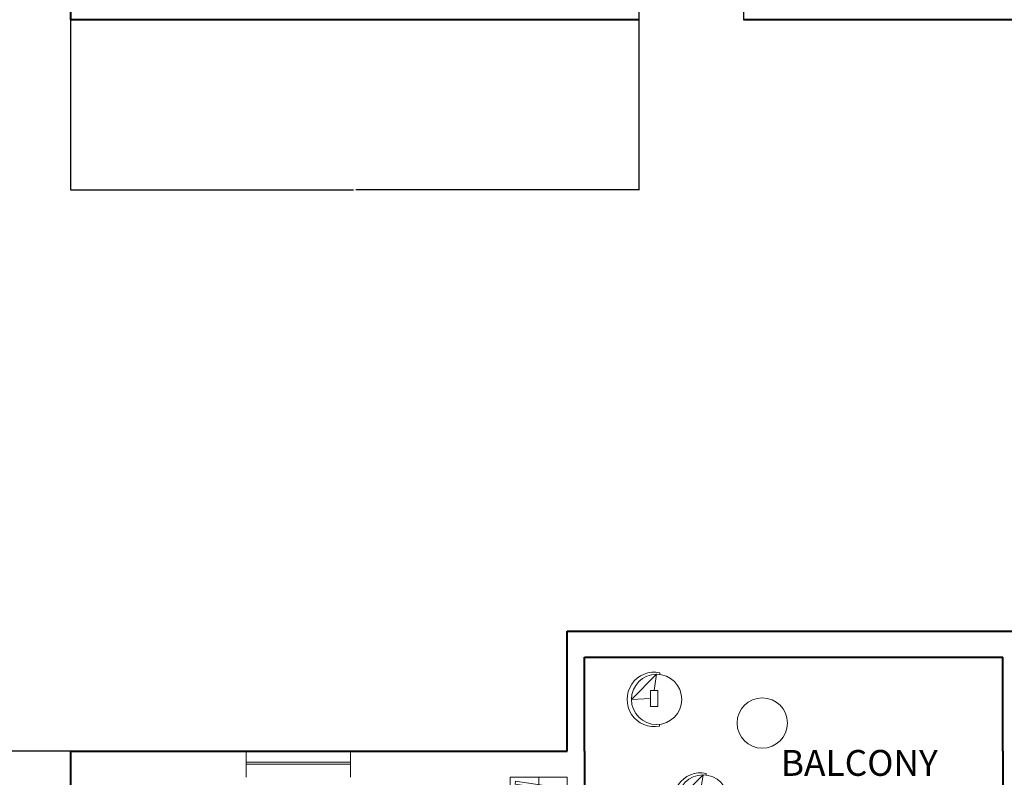
# Model space of a CAD drawing. Units: inches. Extents: x -46 to 1145, y -527 to 760.
# Tile 21 of 57: x 573 to 912, y -39 to 222. Entities that reach past the tile are written whole.
import ezdxf

# ---------------------------------------------------------------- set-up
doc = ezdxf.new("R2010")
doc.units = ezdxf.units.IN
doc.header["$MEASUREMENT"] = 0
for name, color, linetype, lineweight in [('A-ANNO-DIMS', 2, 'Continuous', 18), ('A-AREA-IDEN', 1, 'Continuous', 18), ('A-FLOR-CASE', 32, 'Continuous', 18), ('A-FURN', 2, 'Continuous', 13), ('C-SITE', 7, 'Continuous', 30), ('DOORS', 3, 'Continuous', 25), ('WALLS', 4, 'Continuous', 40), ('WINDOWS', 240, 'Continuous', 20)]:
    doc.layers.add(name, color=color, linetype=linetype, lineweight=lineweight)
doc.styles.get("Standard").update_dxf_attribs({"font": 'arial.ttf'})
doc.dimstyles.get("Standard").update_dxf_attribs({"dimtxt": 0.18, "dimasz": 0.18, "dimexe": 0.18, "dimexo": 0.0625, "dimgap": 0.09, "dimtad": 0, "dimtih": 1, "dimtoh": 1, "dimdec": 0, "dimzin": 0, "dimdsep": 46, "dimlunit": 3, "dimtxsty": 'Standard', "dimcen": 0.09, "dimadec": 0, "dimazin": 0, "dimtfac": 1, "dimtdec": 0, "dimtofl": 0, "dimtmove": 0, "dimatfit": 3, "dimfxl": 1, "dimtolj": 1, "dimtzin": 0, "dimarcsym": 0})

# ---------------------------------------------------------------- blocks, each defined once
blk = doc.blocks.new('*U2')
for p, q in [((0, 0), (0, -6)), ((40, 0), (40, -6))]:
    blk.add_line(p, q)
blk.add_lwpolyline([(0, 0), (0, 40), (1.75, 40), (1.75, 0)], close=True)
blk.add_arc((0, 0), 40, 0, 90)
blk = doc.blocks.new('WARDROBE')
blk.add_line((9.78, 0), (9.78, 83.25))
for points in [[(19.56, 0), (0, 0), (0, 83.25), (19.56, 83.25)], [(17.74, 78.49), (1.66, 80.88), (1.8, 81.87), (17.88, 79.48)], [(15.55, 76.35), (0.49, 70.23), (0.11, 71.16), (15.17, 77.28)], [(18.43, 71.4), (2.35, 73.79), (2.5, 74.78), (18.58, 72.39)], [(16.47, 65.03), (0.39, 67.42), (0.54, 68.41), (16.62, 66.02)], [(15.79, 61), (0.73, 54.88), (0.35, 55.81), (15.41, 61.93)], [(18.43, 57.62), (2.35, 60.01), (2.5, 61), (18.58, 58.61)], [(16.71, 49.68), (0.63, 52.07), (0.78, 53.06), (16.86, 50.67)], [(16.22, 45.12), (1.16, 39), (0.78, 39.93), (15.84, 46.05)], [(18.77, 41.02), (2.69, 43.41), (2.84, 44.4), (18.92, 42.01)], [(17.14, 33.8), (1.06, 36.19), (1.21, 37.19), (17.29, 34.8)], [(16.65, 30.67), (1.59, 24.55), (1.21, 25.48), (16.27, 31.6)], [(17.52, 26.78), (1.44, 29.17), (1.59, 30.16), (17.67, 27.77)], [(17.57, 19.35), (1.49, 21.74), (1.64, 22.73), (17.72, 20.34)], [(17.08, 15.35), (2.02, 9.23), (1.64, 10.16), (16.7, 16.28)], [(18, 4.03), (1.92, 6.42), (2.07, 7.41), (18.15, 5.03)], [(18.32, 0.98), (2.07, 0.98), (2.07, 1.98), (18.32, 1.98)]]:
    blk.add_lwpolyline(points, close=True)
blk = doc.blocks.new('BALCONY-CHAIR')
for p, q in [((1.49, 9.38), (10.16, 18.05)), ((9.33, 12.41), (10.16, 18.05)), ((11.28, 17.97), (11.28, 18.57)), ((8.08, 9.69), (1.49, 9.38)), ((11.2, 0.17), (11.2, 0.77))]:
    blk.add_line(p, q)
blk.add_lwpolyline([(10.57, 6.97), (8.08, 6.97), (8.08, 12.41), (10.57, 12.41)], close=True)
blk.add_circle((10.16, 9.38), 8.67)
blk.add_arc((9.38, 9.38), 9.38, 78.3491, 281.1485)
blk = doc.blocks.new('WINDOW-36IN')
for p, q in [((0, 4.5), (0, 9)), ((0, 9), (0, 0)), ((36, 9), (36, 0)), ((0, 5.23), (36, 5.23)), ((0, 4.5), (36, 4.5))]:
    blk.add_line(p, q)
blk = doc.blocks.new('*D696')
at = {"layer": 'A-ANNO-DIMS', "color": 0, "lineweight": -2, "transparency": 16777216}
for p, q in [((590.06, 221.46), (590.06, 162.74)), ((785.77, 221.46), (785.77, 162.74)), ((590.24, 162.92), (687.53, 162.92)), ((785.59, 162.92), (688.3, 162.92))]:
    blk.add_line(p, q, dxfattribs=at)
at = {"layer": 'A-ANNO-DIMS', "color": 0, "transparency": 16777216}
for points in [[(590.24, 162.95), (590.24, 162.89), (590.06, 162.92)], [(785.59, 162.95), (785.59, 162.89), (785.77, 162.92)]]:
    blk.add_solid(points, dxfattribs=at)
at = {"layer": 'Defpoints', "color": 0, "transparency": 16777216}
for p in [(590.06, 221.52), (785.77, 221.52), (590.06, 162.92)]:
    blk.add_point(p, dxfattribs=at)
at = {"layer": 'A-ANNO-DIMS', "color": 0, "transparency": 16777216, "insert": (687.92, 162.92), "char_height": 0.18, "attachment_point": 5}
blk.add_mtext('\\A1;195.7', dxfattribs=at)

msp = doc.modelspace()

# ---------------------------------------------------------------- linework, layer by layer
at = {"layer": 'A-FURN'}
msp.add_circle((828.2515, -20.7914), 8.6686, dxfattribs=at)
at = {"layer": 'C-SITE'}
msp.add_line((590.0637, -30.4824), (189.5637, -30.4824), dxfattribs=at)
at = {"layer": 'WALLS'}
for p, q in [((590.0637, 659.5176), (590.0637, 221.5176)), ((785.7731, 221.5176), (590.0637, 221.5176)), ((1086.5637, 221.5176), (821.7731, 221.5176)), ((761.0637, -30.4824), (761.0637, 10.8886)), ((761.0637, 10.8886), (767.0637, 10.8886)), ((767.0637, 10.8886), (917.0637, 10.8886)), ((767.0637, 1.8886), (911.0637, 1.8886)), ((767.0637, -30.4824), (767.0637, 1.8886)), ((911.0637, -30.4824), (911.0637, 1.8886)), ((590.0637, -30.4824), (590.0637, -468.4824)), ((590.0637, -30.4824), (761.0637, -30.4824)), ((767.0637, -30.4824), (767.0637, -189.4824)), ((911.0637, -30.4824), (911.0637, -68.1114))]:
    msp.add_line(p, q, dxfattribs=at)

# ---------------------------------------------------------------- block references
at = {"layer": 'A-FLOR-CASE'}
msp.add_blockref('WARDROBE', (741.504, -122.728), dxfattribs=at)
at = {"layer": 'A-FURN'}
for p in [(781.715, -22.034), (797.7165, -56.7085)]:
    msp.add_blockref('BALCONY-CHAIR', p, dxfattribs=at)
at = {"layer": 'DOORS', "xscale": 0.9, "yscale": 0.9, "zscale": 0.9}
msp.add_blockref('*U2', (785.7731, 226.9176), dxfattribs=at)
at = {"layer": 'WINDOWS'}
msp.add_blockref('WINDOW-36IN', (650.495, -39.482), dxfattribs=at)

# ---------------------------------------------------------------- texts
at = {"layer": 'A-AREA-IDEN'}
msp.add_text(' BALCONY', height=8.92326, dxfattribs=at).set_placement((831.917, -38.979))

# ---------------------------------------------------------------- dimensions: what is measured, and where the dimension line sits
at = {"layer": 'A-ANNO-DIMS'}
dim = msp.add_linear_dim(base=(590.0637, 162.9176), p1=(785.7731, 221.5176), p2=(590.0637, 221.5176), angle=180, dimstyle='Standard', override={"dimdec": 1, "dimlfac": 1, "dimrnd": 0, "dimzin": 0, "dimdsep": 46, "dimlunit": 2}, dxfattribs=at)
dim.commit()
dim.dimension.update_dxf_attribs({"geometry": '*D696', "text_midpoint": (687.9184, 162.9176)})

doc.saveas('drawing.dxf')
